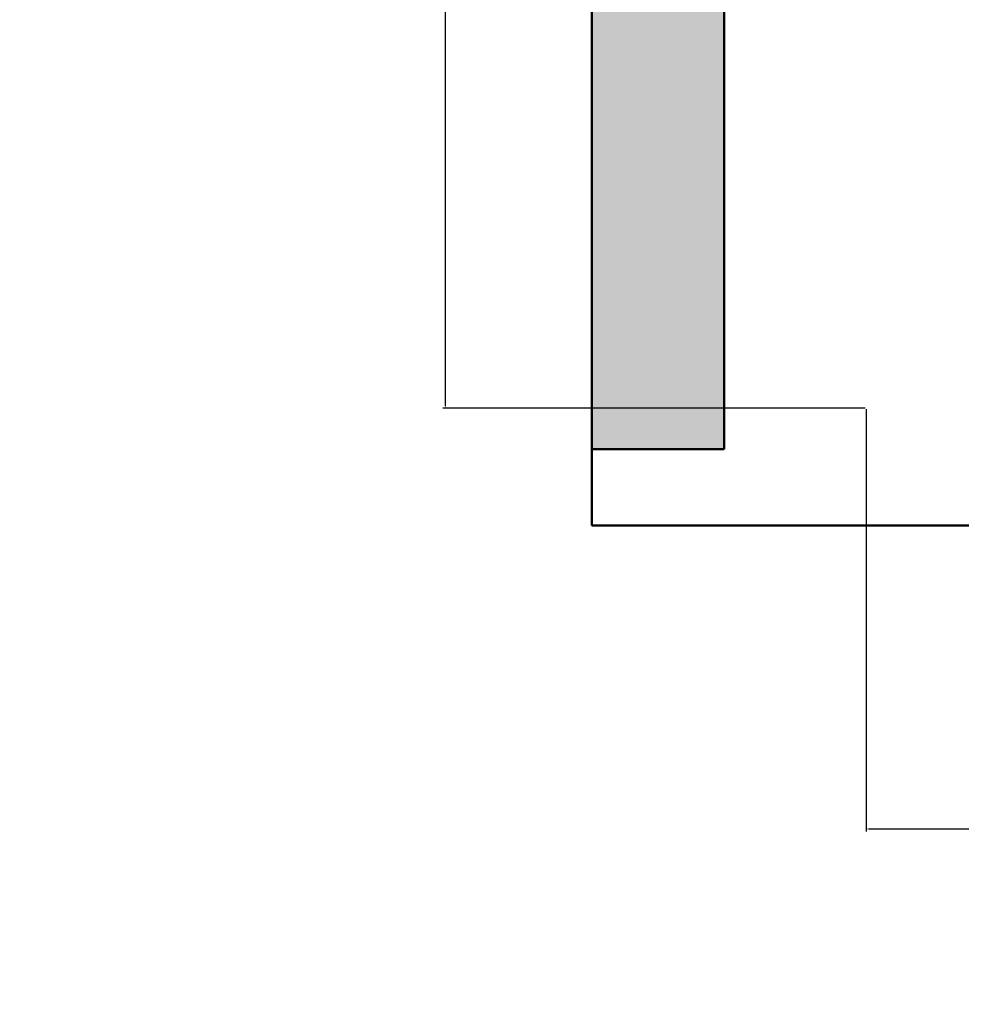
# Model space of a CAD drawing. Units: inches. Extents: x 22042254 to 25404563, y 17568978 to 17626777.
# Tile 19 of 45: x 22179745 to 22179809, y 17626160 to 17626227. Entities that reach past the tile are written whole.
import ezdxf

# ---------------------------------------------------------------- set-up
doc = ezdxf.new("R2010")
doc.units = ezdxf.units.IN
doc.header["$MEASUREMENT"] = 0
for name, color, linetype, lineweight in [('A-ANNO-DIMS', 2, 'Continuous', 18), ('A-WALL-PATT', 244, 'Continuous', 13), ('walls', 252, 'Continuous', 50)]:
    doc.layers.add(name, color=color, linetype=linetype, lineweight=lineweight)
doc.styles.get("Standard").update_dxf_attribs({"font": 'arial.ttf'})
doc.dimstyles.get("Standard").update_dxf_attribs({"dimtxt": 8, "dimasz": 0.18, "dimexe": 0.18, "dimexo": 0.0625, "dimgap": 0.09, "dimtad": 0, "dimtih": 1, "dimtoh": 1, "dimzin": 0, "dimdsep": 46, "dimlunit": 3, "dimtxsty": 'Standard', "dimcen": 0.09, "dimadec": 0, "dimazin": 0, "dimtfac": 1, "dimtofl": 0, "dimtmove": 0, "dimatfit": 3, "dimfxl": 1, "dimtolj": 1, "dimtzin": 0, "dimarcsym": 0})

# ---------------------------------------------------------------- blocks, each defined once
blk = doc.blocks.new('*D58')
at = {"layer": 'A-ANNO-DIMS', "color": 0, "lineweight": -2, "transparency": 16777216}
for p, q in [((22179802.339, 17626391.376), (22179773.599, 17626391.376)), ((22179773.779, 17626391.196), (22179773.779, 17626300.194)), ((22179773.779, 17626200.739), (22179773.779, 17626291.741)), ((22179802.339, 17626200.559), (22179773.599, 17626200.559))]:
    blk.add_line(p, q, dxfattribs=at)
at = {"layer": 'A-ANNO-DIMS', "color": 0, "transparency": 16777216}
for points in [[(22179773.749, 17626391.196), (22179773.809, 17626391.196), (22179773.779, 17626391.376)], [(22179773.749, 17626200.739), (22179773.809, 17626200.739), (22179773.779, 17626200.559)]]:
    blk.add_solid(points, dxfattribs=at)
at = {"layer": 'Defpoints', "color": 0, "transparency": 16777216}
for p in [(22179802.402, 17626391.376), (22179773.779, 17626200.559), (22179802.402, 17626200.559)]:
    blk.add_point(p, dxfattribs=at)
at = {"layer": 'A-ANNO-DIMS', "color": 0, "transparency": 16777216, "insert": (22179773.779, 17626295.968), "char_height": 8, "attachment_point": 5}
blk.add_mtext('\\A1;CAR 15\'-11"', dxfattribs=at)
blk = doc.blocks.new('*D59')
at = {"layer": 'A-ANNO-DIMS', "color": 0, "lineweight": -2, "transparency": 16777216}
for p, q in [((22179802.402, 17626200.497), (22179802.402, 17626171.756)), ((22179895.926, 17626200.497), (22179895.926, 17626171.756)), ((22179802.582, 17626171.936), (22179829.153, 17626171.936)), ((22179895.746, 17626171.936), (22179869.175, 17626171.936))]:
    blk.add_line(p, q, dxfattribs=at)
at = {"layer": 'A-ANNO-DIMS', "color": 0, "transparency": 16777216}
for points in [[(22179802.582, 17626171.966), (22179802.582, 17626171.906), (22179802.402, 17626171.936)], [(22179895.746, 17626171.966), (22179895.746, 17626171.906), (22179895.926, 17626171.936)]]:
    blk.add_solid(points, dxfattribs=at)
at = {"layer": 'Defpoints', "color": 0, "transparency": 16777216}
for p in [(22179802.402, 17626200.559), (22179895.926, 17626200.559), (22179895.926, 17626171.936)]:
    blk.add_point(p, dxfattribs=at)
at = {"layer": 'A-ANNO-DIMS', "color": 0, "transparency": 16777216, "insert": (22179849.164, 17626171.936), "char_height": 8, "attachment_point": 5}
blk.add_mtext('\\A1;7\'-9 1/2"', dxfattribs=at)

msp = doc.modelspace()

# ---------------------------------------------------------------- hatches: boundary and pattern name
at = {"layer": 'A-WALL-PATT'}
h = msp.add_hatch(color=256, dxfattribs=at)
h.dxf.hatch_style = 1
h.paths.add_polyline_path([(22179792.734, 17626580.28), (22179888.734, 17626580.28), (22179888.734, 17626559.623), (22179893.234, 17626559.623), (22179893.234, 17626580.28), (22179900.438, 17626580.28), (22179900.438, 17626584.78), (22179792.734, 17626584.78), (22179792.734, 17626728.78), (22180134.734, 17626728.78), (22180134.734, 17626584.78), (22180035.602, 17626584.78), (22180004.432, 17626584.78), (22180001.734, 17626584.78), (22180001.734, 17626580.28), (22180134.734, 17626580.28), (22180134.734, 17626404.28), (22180064.487, 17626404.28), (22180064.487, 17626399.78), (22180134.734, 17626399.78), (22180134.734, 17626197.78), (22180143.734, 17626197.78), (22180143.734, 17626737.78), (22179783.734, 17626737.78), (22179783.734, 17626197.78), (22179792.734, 17626197.78), (22179792.734, 17626394.78), (22179936.734, 17626394.78), (22179936.734, 17626383.208), (22179941.234, 17626383.208), (22179941.234, 17626532.28), (22179927.066, 17626532.28), (22179927.066, 17626527.78), (22179928.072, 17626527.78), (22179936.734, 17626527.78), (22179936.734, 17626403.78), (22179792.734, 17626403.78), (22179792.734, 17626527.78), (22179905.094, 17626527.78), (22179905.094, 17626532.28), (22179792.734, 17626532.28)])

# ---------------------------------------------------------------- linework, layer by layer
at = {"layer": 'walls'}
for p, q in [((22179783.734, 17626197.78), (22179783.734, 17626737.78)), ((22179792.734, 17626197.78), (22179792.734, 17626394.78)), ((22179783.734, 17626192.584), (22179783.734, 17626202.976)), ((22179792.734, 17626197.78), (22179783.734, 17626197.78)), ((22179783.734, 17626192.584), (22179936.734, 17626192.584))]:
    msp.add_line(p, q, dxfattribs=at)

# ---------------------------------------------------------------- dimensions: what is measured, and where the dimension line sits
at = {"layer": 'A-ANNO-DIMS'}
dim = msp.add_linear_dim(base=(22179773.779, 17626200.559), p1=(22179802.402, 17626391.376), p2=(22179802.402, 17626200.559), angle=270, text='CAR <>', dimstyle='Standard', override={"dimdec": 1, "dimlfac": 1, "dimrnd": 0, "dimzin": 1, "dimdsep": 46, "dimlunit": 4, "dimfrac": 2}, dxfattribs=at)
dim.commit()
dim.dimension.update_dxf_attribs({"geometry": '*D58', "text_midpoint": (22179773.779, 17626295.968)})
dim = msp.add_linear_dim(base=(22179895.926, 17626171.936), p1=(22179802.402, 17626200.559), p2=(22179895.926, 17626200.559), dimstyle='Standard', override={"dimdec": 1, "dimlfac": 1, "dimrnd": 0, "dimzin": 1, "dimdsep": 46, "dimlunit": 4, "dimfrac": 2}, dxfattribs=at)
dim.commit()
dim.dimension.update_dxf_attribs({"geometry": '*D59', "text_midpoint": (22179849.164, 17626171.936)})

doc.saveas('drawing.dxf')
